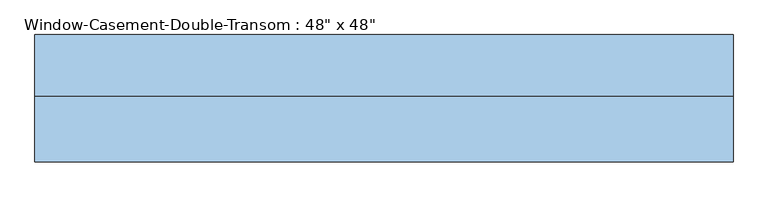
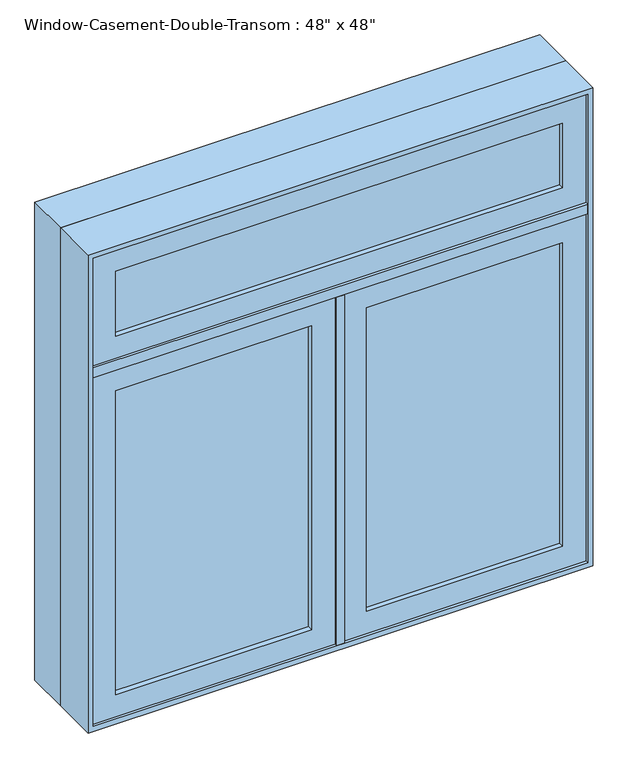
"""IFC4 building model written with IfcOpenShell, lengths in millimetres: window geometry."""

from ifc_helpers import new_model, si_unit, frame, origin, place, context, project, spatial, polyline, outline, extrude, faceted_brep, source, transform, mapped, element, save


def window_3911def3(model_context):
    return source(origin(), model_context, "Body", "SolidModel", [
        faceted_brep([(577.85, -69.85, 2101.85), (-577.85, -69.85, 2101.85), (-577.85, -6.35, 2101.85), (577.85, -6.35, 2101.85), (596.9, -120.65, 2120.9), (-596.9, -120.65, 2120.9), (-596.9, -69.85, 2120.9), (596.9, -69.85, 2120.9), (609.6, -6.35, 2133.6), (-609.6, -6.35, 2133.6), (-609.6, -120.65, 2133.6), (609.6, -120.65, 2133.6), (-577.85, -69.85, 946.15), (-577.85, -6.35, 946.15), (-596.9, -120.65, 927.1), (-596.9, -69.85, 927.1), (-609.6, -6.35, 914.4), (-609.6, -120.65, 914.4), (577.85, -69.85, 946.15), (577.85, -6.35, 946.15), (596.9, -120.65, 927.1), (596.9, -69.85, 927.1), (609.6, -6.35, 914.4), (609.6, -120.65, 914.4)], [[[0, 1, 2, 3]], [[4, 5, 6, 7]], [[8, 9, 10, 11]], [[1, 12, 13, 2]], [[5, 14, 15, 6]], [[9, 16, 17, 10]], [[12, 18, 19, 13]], [[14, 20, 21, 15]], [[16, 22, 23, 17]], [[9, 8, 22, 16], [3, 2, 13, 19]], [[18, 0, 3, 19]], [[7, 6, 15, 21], [1, 0, 18, 12]], [[20, 4, 7, 21]], [[22, 8, 11, 23]], [[11, 10, 17, 23], [5, 4, 20, 14]]]),
        extrude(outline(polyline([(2133.6, -609.6), (914.4, -609.6), (914.4, 609.6), (2133.6, 609.6), (2133.6, -609.6)]), holes=[polyline([(2114.55, 590.55), (933.45, 590.55), (933.45, -590.55), (2114.55, -590.55), (2114.55, 590.55)])]), frame((0.0, -6.35, 0.0), z_axis=(0.0, 1.0, 0.0), x_axis=(0.0, 0.0, 1.0)), (0.0, 0.0, 1.0), 107.95),
        extrude(outline(polyline([(927.1, 9.525), (927.1, 596.9), (1816.1, 596.9), (1816.1, 9.525), (927.1, 9.525)]), holes=[polyline([(984.25, 539.75), (984.25, 66.675), (1758.95, 66.675), (1758.95, 539.75), (984.25, 539.75)])]), frame((0.0, -114.3, 0.0), z_axis=(0.0, 1.0, 0.0), x_axis=(0.0, 0.0, 1.0)), (0.0, 0.0, 1.0), 44.45),
        extrude(outline(polyline([(1816.1, -9.525), (1816.1, -596.9), (927.1, -596.9), (927.1, -9.525), (1816.1, -9.525)]), holes=[polyline([(1758.95, -539.75), (1758.95, -66.675), (984.25, -66.675), (984.25, -539.75), (1758.95, -539.75)])]), frame((0.0, -114.3, 0.0), z_axis=(0.0, 1.0, 0.0), x_axis=(0.0, 0.0, 1.0)), (0.0, 0.0, 1.0), 44.45),
        extrude(outline(polyline([(539.75, -101.6), (66.675, -101.6), (66.675, -95.25), (539.75, -95.25), (539.75, -101.6)])), frame((0.0, 0.0, 984.25), z_axis=(0.0, 0.0, 1.0), x_axis=(1.0, 0.0, 0.0)), (0.0, 0.0, 1.0), 774.7),
        extrude(outline(polyline([(66.675, -82.55), (539.75, -82.55), (539.75, -88.9), (66.675, -88.9), (66.675, -82.55)])), frame((0.0, 0.0, 984.25), z_axis=(0.0, 0.0, 1.0), x_axis=(1.0, 0.0, 0.0)), (0.0, 0.0, 1.0), 774.7),
        extrude(outline(polyline([(-66.675, -101.6), (-539.75, -101.6), (-539.75, -95.25), (-66.675, -95.25), (-66.675, -101.6)])), frame((0.0, 0.0, 984.25), z_axis=(0.0, 0.0, 1.0), x_axis=(1.0, 0.0, 0.0)), (0.0, 0.0, 1.0), 774.7),
        extrude(outline(polyline([(-539.75, -82.55), (-66.675, -82.55), (-66.675, -88.9), (-539.75, -88.9), (-539.75, -82.55)])), frame((0.0, 0.0, 984.25), z_axis=(0.0, 0.0, 1.0), x_axis=(1.0, 0.0, 0.0)), (0.0, 0.0, 1.0), 774.7),
        faceted_brep([(9.525, -120.65, 1816.1), (9.525, -69.85, 1816.1), (30.1625, -69.85, 1816.1), (30.1625, -6.35, 1816.1), (-30.1625, -6.35, 1816.1), (-30.1625, -69.85, 1816.1), (-9.525, -69.85, 1816.1), (-9.525, -120.65, 1816.1), (9.525, -120.65, 927.1), (-9.525, -120.65, 927.1), (-9.525, -69.85, 927.1), (9.525, -69.85, 927.1), (-9.525, -69.85, 946.15), (-30.1625, -69.85, 946.15), (-30.1625, -6.35, 946.15), (30.1625, -6.35, 946.15), (30.1625, -69.85, 946.15), (9.525, -69.85, 946.15)], [[[0, 1, 2, 3, 4, 5, 6, 7]], [[8, 9, 10, 11]], [[7, 9, 8, 0]], [[6, 12, 10, 9, 7]], [[5, 13, 12, 6]], [[4, 14, 13, 5]], [[3, 15, 14, 4]], [[2, 16, 15, 3]], [[1, 17, 16, 2]], [[0, 8, 11, 17, 1]], [[17, 11, 10, 12]], [[12, 13, 14, 15, 16, 17]]]),
        extrude(outline(polyline([(539.75, -101.6), (-539.75, -101.6), (-539.75, -95.25), (539.75, -95.25), (539.75, -101.6)])), frame((0.0, 0.0, 1898.65), z_axis=(0.0, 0.0, 1.0), x_axis=(1.0, 0.0, 0.0)), (0.0, 0.0, 1.0), 165.1),
        extrude(outline(polyline([(-539.75, -82.55), (539.75, -82.55), (539.75, -88.9), (-539.75, -88.9), (-539.75, -82.55)])), frame((0.0, 0.0, 1898.65), z_axis=(0.0, 0.0, 1.0), x_axis=(1.0, 0.0, 0.0)), (0.0, 0.0, 1.0), 165.1),
        extrude(outline(polyline([(596.9, -120.65), (-596.9, -120.65), (-596.9, -69.85), (-577.85, -69.85), (-577.85, -6.35), (577.85, -6.35), (577.85, -69.85), (596.9, -69.85), (596.9, -120.65)])), frame((0.0, 0.0, 1816.1), z_axis=(0.0, 0.0, 1.0), x_axis=(1.0, 0.0, 0.0)), (0.0, 0.0, 1.0), 25.4),
        extrude(outline(polyline([(2120.9, 596.9), (2120.9, -596.9), (1841.5, -596.9), (1841.5, 596.9), (2120.9, 596.9)]), holes=[polyline([(2063.75, -539.75), (2063.75, 539.75), (1898.65, 539.75), (1898.65, -539.75), (2063.75, -539.75)])]), frame((0.0, -114.3, 0.0), z_axis=(0.0, 1.0, 0.0), x_axis=(0.0, 0.0, 1.0)), (0.0, 0.0, 1.0), 44.45),
    ])


if __name__ == "__main__":
    model = new_model("IFC4")
    model_context = context("Model", 3, world=origin())
    ifc_project = project(units=[si_unit("LENGTHUNIT", "METRE", prefix="MILLI")], contexts=[model_context])
    site = spatial("IfcSite", under=ifc_project)
    building = spatial("IfcBuilding", under=site)
    placement = place(None, origin())
    window_shape = window_3911def3(model_context)
    element("IfcWindow", 1, ObjectType="Window-Casement-Double-Transom : 48\" x 48\"", at=placement, inside=building, context=model_context, shape_type="MappedRepresentation", body=[
        mapped(window_shape, transform((0.0, 0.0, 0.0), x_axis=(1.0, 0.0, 0.0), y_axis=(0.0, 1.0, 0.0), z_axis=(0.0, 0.0, 1.0))),
    ])
    save(model, "model.ifc")

# Revit data of these elements
# Type "Window-Casement-Double-Transom : 48\" x 48\""
#   Type Mark = "18"
#   Fire Rating = "0.5h"
#   Assembly Code = "B2020100"
#   Analytic Construction = "Double glazing - domestic"
#   Window Inset [instance default] = 0' - 0"
#   Wall Thickness [instance default] = 0' - 6"
#   Interior Wall Closure [instance default] = 0' - 2 1/4"
#   Half Width = 2' - 0"
#   Visual Light Transmittance = 0.81
#   Transom Height = 1' - 0"
#   Thermal Resistance (R) = 1.8146 (h·ft²·°F)/BTU
#   Solar Heat Gain Coefficient = 0.76
#   Rough Width = 4' - 0 1/2"
#   Rough Height = 4' - 0 1/2"
#   Open Window Height = 3' - 0"
#   Height = 4' - 0"
#   Heat Transfer Coefficient (U) = 0.5511 BTU/(h·ft²·°F)
#   Frame Extension [instance default] = 0' - 0 1/4"
#   Exterior Wall Closure [instance default] = 0' - 1 1/4"
#   Extension Jamb [instance default] = 0' - 2 1/4"
#   Default Sill Height = 3' - 0"
#   Width = 4' - 0"
#   Muntin Visibility = yes
#   Interior Trim Visibility [instance default] = yes
#   Exterior Trim Visibility [instance default] = yes
#   Extension Jamb Visibility [instance default] = yes
#   Interior Trim Material = Wood - Stained
#   Muntin Pattern = Muntin Pattern_2x2 : Muntin Pattern_2x2
#   Interior Trim = Trim-Window-Interior-Flat : Picture Frame
#   Interior Frame Material = Wood - Stained
#   Glass Panel Material = Glass
#   Exterior Trim Material = Clad - White
#   Exterior Trim = Trim-Window-Exterior-Flat : with Sill
#   Exterior Frame Material = Clad - White
#   Wall Closure = (empty or 0)
# Element 1 (IfcWindow, "Window-Casement-Double-Transom : 48\" x 48\"")
#   Wall Thickness = 0' - 8"
#   Extension Jamb = 0' - 4 1/4"
#   Materials on its faces: "Wood - Stained", "Glass", "Clad - White"
# Materials
#   "Wood - Stained": class "Wood", colour RGB 224 178 126, transparency 0, Cost = 0
#   "Glass": class "Glass", colour RGB 0 128 192, transparency 0.75, Description = "Soda Lime Glass", Cost = 0
#   "Clad - White": class "Wood", colour RGB 242 242 238, transparency 0, Cost = 0
